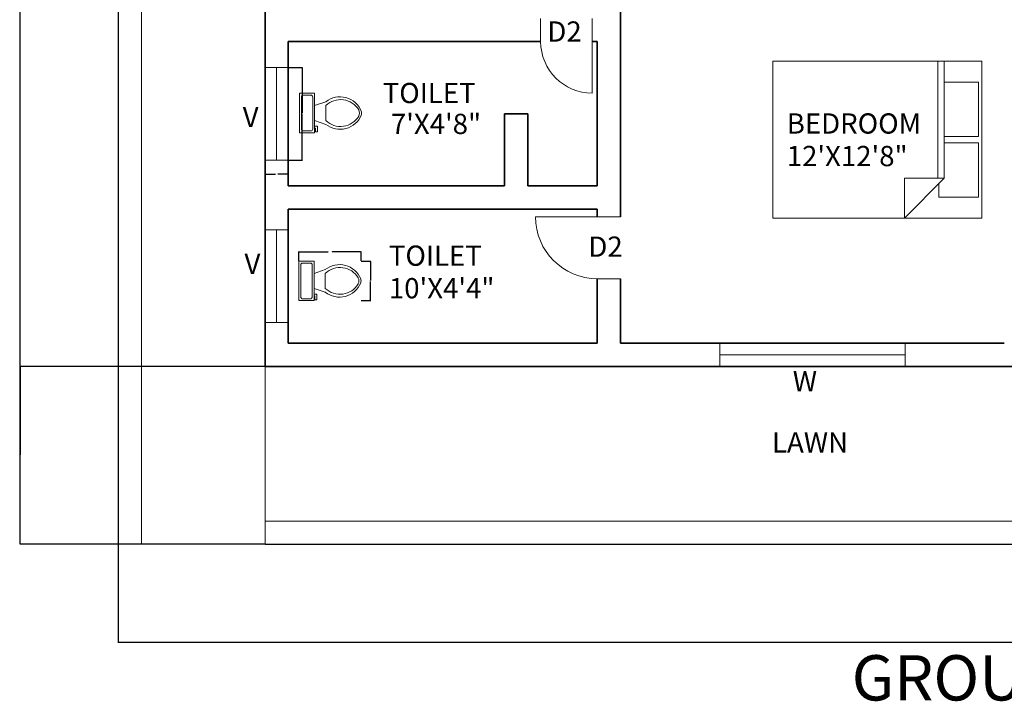
# Model space of a CAD drawing. Units: feet. Extents: x 2219 to 3039, y 1768 to 2369.
# Tile 1 of 16: x 2219 to 2601, y 1768 to 2032. Entities that reach past the tile are written whole.
import ezdxf

# ---------------------------------------------------------------- set-up
doc = ezdxf.new("R2010")
doc.units = ezdxf.units.FT
for name, color, linetype, lineweight in [('A-ANNO-DIMS', 2, 'Continuous', 18), ('A-ANNO-TEXT', 7, 'Continuous', 18), ('A-ANNO-TITL', 7, 'Continuous', 35), ('A-AREA-IDEN', 7, 'Continuous', 18), ('A-DOOR', 4, 'Continuous', 20), ('A-FLOR-FIXT', 9, 'Continuous', 18), ('A-FURN', 8, 'Continuous', 18), ('A-GLAZ', 4, 'Continuous', 18), ('A-WALL', 7, 'Continuous', 35), ('C-PROP', 7, 'Continuous', 30), ('C-SITE', 3, 'Continuous', 20)]:
    doc.layers.add(name, color=color, linetype=linetype, lineweight=lineweight)
doc.styles.get("Standard").update_dxf_attribs({"font": 'arial.ttf'})
doc.dimstyles.get("Standard").update_dxf_attribs({"dimtxt": 0.18, "dimasz": 0.18, "dimexe": 0.18, "dimexo": 0.0625, "dimgap": 0.09, "dimtad": 0, "dimtih": 1, "dimtoh": 1, "dimdec": 4, "dimzin": 0, "dimdsep": 46, "dimtxsty": 'Standard', "dimcen": 0.09, "dimadec": 0, "dimazin": 0, "dimtfac": 1, "dimtdec": 4, "dimtofl": 0, "dimtmove": 0, "dimatfit": 3, "dimfxl": 1, "dimtolj": 1, "dimtzin": 0, "dimarcsym": 0})

# ---------------------------------------------------------------- blocks, each defined once
blk = doc.blocks.new('Bed - Queen')
for p, q in [((0, -80.00003), (0, 0)), ((0, 0), (59.99999, 0)), ((59.99999, 0), (59.99999, -80.00003)), ((7.99999, -1.2), (28.79998, -1.2)), ((7.99999, -14.4), (7.99999, -1.2)), ((28.79998, -1.2), (28.79998, -14.4)), ((31.19999, -1.2), (51.99999, -1.2)), ((31.19999, -14.4), (31.19999, -1.2)), ((51.99999, -1.2), (51.99999, -16.4)), ((0, -14.4), (44.8, -14.4)), ((59.99999, -29.6), (44.8, -14.4)), ((44.8, -14.4), (44.8, -29.6)), ((44.8, -16.8), (0, -16.8)), ((51.99999, -16.4), (46.79936, -16.4)), ((44.8, -29.6), (59.99999, -29.6)), ((59.99999, -80.00003), (0, -80.00003))]:
    blk.add_line(p, q)
blk = doc.blocks.new('Toilet - top')
for p, q in [((9.5, -6), (9.5, -2)), ((-10, -8.5), (-8, -8.5)), ((-10, -9.5), (-10, -8.5)), ((-7, -9.5), (-10, -9.5)), ((-8, -8.5), (-8, -8)), ((-7, -8), (-7, -9.5)), ((-4, -8), (-6, -14)), ((4, -8), (6, -14)), ((4, -14), (-4, -14))]:
    blk.add_line(p, q)
blk.add_lwpolyline([(10.5, -8), (10.5, 0), (-10.5, 0), (-10.5, -8)], close=True)
for points in [[(-9.5, -2), (-9.5, -6)], [(8.5, -1), (-8.5, -1)], [(-8.5, -7), (8.5, -7)]]:
    blk.add_lwpolyline(points)
for centre, radius, start, end in [((-8.62, -1.88), 0.884, 81.8699, 188.1301), ((8.62, -1.88), 0.884, 351.8699, 98.1301), ((-8.62, -6.12), 0.884, 171.8699, 278.1301), ((8.62, -6.12), 0.884, 261.8699, 8.1301), ((3.52, -21.58), 12.17, 141.4691, 247.9714), ((4.2, -21.82), 11.33, 136.3677, 238.9468), ((-3.52, -21.58), 12.17, 292.0284, 38.5307), ((-4.2, -21.82), 11.33, 301.053, 43.6321), ((0, -27.88), 4, 245.7318, 294.2682), ((0, -29), 4, 254.8605, 285.1395)]:
    blk.add_arc(centre, radius, start, end)
blk = doc.blocks.new('DOOR-24-INTEGRAL-JAMB')
for p, q in [((9, 24), (0, 24)), ((33, 0), (0, 0))]:
    blk.add_line(p, q)
blk.add_arc((9, 0), 24, 0, 90)
blk = doc.blocks.new('DOOR-20')
for p, q in [((0, 29), (0, 0)), ((20, 9), (20, 0))]:
    blk.add_line(p, q)
blk.add_arc((0, 9), 20, 0, 90)
blk = doc.blocks.new('WINDOW-72')
for p, q in [((9, 72), (0, 72)), ((4.5, 72), (4.5, 0)), ((9, 0), (0, 0))]:
    blk.add_line(p, q)
blk = doc.blocks.new('VENT-WINDOW-36')
for p, q in [((0, 36), (9, 36)), ((4.5, 36), (4.5, 0)), ((0, 0), (9, 0))]:
    blk.add_line(p, q)
blk = doc.blocks.new('*D18')
at = {"layer": 'A-ANNO-DIMS', "color": 0, "lineweight": -2, "transparency": 16777216}
for p, q in [((2327.57, 1938.8), (2327.57, 1942.54)), ((2327.75, 1942.36), (2338.85, 1942.36)), ((2351.5, 1942.36), (2340.4, 1942.36)), ((2351.68, 1938.8), (2351.68, 1942.54))]:
    blk.add_line(p, q, dxfattribs=at)
at = {"layer": 'A-ANNO-DIMS', "color": 0, "transparency": 16777216}
for points in [[(2327.75, 1942.39), (2327.75, 1942.33), (2327.57, 1942.36)], [(2351.5, 1942.39), (2351.5, 1942.33), (2351.68, 1942.36)]]:
    blk.add_solid(points, dxfattribs=at)
at = {"layer": 'Defpoints', "color": 0, "transparency": 16777216}
for p in [(2327.57, 1942.36), (2327.57, 1938.74), (2351.68, 1938.74)]:
    blk.add_point(p, dxfattribs=at)
at = {"layer": 'A-ANNO-DIMS', "color": 0, "transparency": 16777216, "insert": (2339.63, 1942.36), "char_height": 0.18, "attachment_point": 5}
blk.add_mtext('\\A1;WC 24 TYP.', dxfattribs=at)
blk = doc.blocks.new('*D19')
at = {"layer": 'A-ANNO-DIMS', "color": 0, "lineweight": -2, "transparency": 16777216}
for p, q in [((2351.75, 1938.74), (2355.48, 1938.74)), ((2355.3, 1938.56), (2355.3, 1931.26)), ((2355.3, 1923.6), (2355.3, 1930.9)), ((2351.75, 1923.42), (2355.48, 1923.42))]:
    blk.add_line(p, q, dxfattribs=at)
at = {"layer": 'A-ANNO-DIMS', "color": 0, "transparency": 16777216}
for points in [[(2355.27, 1938.56), (2355.33, 1938.56), (2355.3, 1938.74)], [(2355.27, 1923.6), (2355.33, 1923.6), (2355.3, 1923.42)]]:
    blk.add_solid(points, dxfattribs=at)
at = {"layer": 'Defpoints', "color": 0, "transparency": 16777216}
for p in [(2351.68, 1938.74), (2355.3, 1938.74), (2351.68, 1923.42)]:
    blk.add_point(p, dxfattribs=at)
at = {"layer": 'A-ANNO-DIMS', "color": 0, "transparency": 16777216, "insert": (2355.3, 1931.08), "char_height": 0.18, "attachment_point": 5}
blk.add_mtext('\\A1;15 TYP.', dxfattribs=at)
blk = doc.blocks.new('*D38')
at = {"layer": 'A-ANNO-DIMS', "color": 0, "lineweight": -2, "transparency": 16777216}
for p, q in [((2323.46, 2013.92), (2328.98, 2013.92)), ((2328.8, 2013.74), (2328.8, 1996.11)), ((2328.8, 1978.1), (2328.8, 1995.74)), ((2323.46, 1977.92), (2328.98, 1977.92))]:
    blk.add_line(p, q, dxfattribs=at)
at = {"layer": 'A-ANNO-DIMS', "color": 0, "transparency": 16777216}
for points in [[(2328.77, 2013.74), (2328.83, 2013.74), (2328.8, 2013.92)], [(2328.77, 1978.1), (2328.83, 1978.1), (2328.8, 1977.92)]]:
    blk.add_solid(points, dxfattribs=at)
at = {"layer": 'Defpoints', "color": 0, "transparency": 16777216}
for p in [(2323.4, 2013.92), (2328.8, 2013.92), (2323.4, 1977.92)]:
    blk.add_point(p, dxfattribs=at)
at = {"layer": 'A-ANNO-DIMS', "color": 0, "transparency": 16777216, "insert": (2328.8, 1995.92), "char_height": 0.18, "attachment_point": 5}
blk.add_mtext('\\A1;VENT WINDOW 36 TYP.', dxfattribs=at)
blk = doc.blocks.new('*D39')
at = {"layer": 'A-ANNO-DIMS', "color": 0, "lineweight": -2, "transparency": 16777216}
for p, q in [((2314.4, 1977.86), (2314.4, 1972.34)), ((2323.4, 1977.86), (2323.4, 1972.34)), ((2314.58, 1972.52), (2318.44, 1972.52)), ((2323.22, 1972.52), (2319.36, 1972.52))]:
    blk.add_line(p, q, dxfattribs=at)
at = {"layer": 'A-ANNO-DIMS', "color": 0, "transparency": 16777216}
for points in [[(2314.58, 1972.55), (2314.58, 1972.49), (2314.4, 1972.52)], [(2323.22, 1972.55), (2323.22, 1972.49), (2323.4, 1972.52)]]:
    blk.add_solid(points, dxfattribs=at)
at = {"layer": 'Defpoints', "color": 0, "transparency": 16777216}
for p in [(2314.4, 1977.92), (2323.4, 1977.92), (2323.4, 1972.52)]:
    blk.add_point(p, dxfattribs=at)
at = {"layer": 'A-ANNO-DIMS', "color": 0, "transparency": 16777216, "insert": (2318.9, 1972.52), "char_height": 0.18, "attachment_point": 5}
blk.add_mtext('\\A1;9 TYP.', dxfattribs=at)
blk = doc.blocks.new('*D46')
at = {"layer": 'A-ANNO-DIMS', "color": 0, "lineweight": -2, "transparency": 16777216}
for p, q in [((2257.4, 1828.86), (2257.4, 1790.69)), ((3000.4, 1828.86), (3000.4, 1790.69)), ((2257.58, 1790.87), (2628.61, 1790.87)), ((3000.22, 1790.87), (2629.19, 1790.87))]:
    blk.add_line(p, q, dxfattribs=at)
at = {"layer": 'A-ANNO-DIMS', "color": 0, "transparency": 16777216}
for points in [[(2257.58, 1790.9), (2257.58, 1790.84), (2257.4, 1790.87)], [(3000.22, 1790.9), (3000.22, 1790.84), (3000.4, 1790.87)]]:
    blk.add_solid(points, dxfattribs=at)
at = {"layer": 'Defpoints', "color": 0, "transparency": 16777216}
for p in [(2257.4, 1828.92), (3000.4, 1828.92), (3000.4, 1790.87)]:
    blk.add_point(p, dxfattribs=at)
at = {"layer": 'A-ANNO-DIMS', "color": 0, "transparency": 16777216, "insert": (2628.9, 1790.87), "char_height": 0.18, "attachment_point": 5}
blk.add_mtext('\\A1;743', dxfattribs=at)
blk = doc.blocks.new('*D47')
at = {"layer": 'A-ANNO-DIMS', "color": 0, "lineweight": -2, "transparency": 16777216}
for p, q in [((2257.34, 2330.92), (2219.17, 2330.92)), ((2219.35, 2330.74), (2219.35, 2080.1)), ((2219.35, 1829.1), (2219.35, 2079.74)), ((2257.34, 1828.92), (2219.17, 1828.92))]:
    blk.add_line(p, q, dxfattribs=at)
at = {"layer": 'A-ANNO-DIMS', "color": 0, "transparency": 16777216}
for points in [[(2219.32, 2330.74), (2219.38, 2330.74), (2219.35, 2330.92)], [(2219.32, 1829.1), (2219.38, 1829.1), (2219.35, 1828.92)]]:
    blk.add_solid(points, dxfattribs=at)
at = {"layer": 'Defpoints', "color": 0, "transparency": 16777216}
for p in [(2219.35, 2330.92), (2257.4, 2330.92), (2257.4, 1828.92)]:
    blk.add_point(p, dxfattribs=at)
at = {"layer": 'A-ANNO-DIMS', "color": 0, "transparency": 16777216, "insert": (2219.35, 2079.92), "char_height": 0.18, "attachment_point": 5}
blk.add_mtext('\\A1;502', dxfattribs=at)
blk = doc.blocks.new('*D48')
at = {"layer": 'A-ANNO-DIMS', "color": 0, "lineweight": -2, "transparency": 16777216}
for p, q in [((2314.34, 1897.92), (2219.17, 1897.92)), ((2219.35, 1897.74), (2219.35, 1863.6)), ((2219.35, 1829.1), (2219.35, 1863.24)), ((2314.34, 1828.92), (2219.17, 1828.92))]:
    blk.add_line(p, q, dxfattribs=at)
at = {"layer": 'A-ANNO-DIMS', "color": 0, "transparency": 16777216}
for points in [[(2219.32, 1897.74), (2219.38, 1897.74), (2219.35, 1897.92)], [(2219.32, 1829.1), (2219.38, 1829.1), (2219.35, 1828.92)]]:
    blk.add_solid(points, dxfattribs=at)
at = {"layer": 'Defpoints', "color": 0, "transparency": 16777216}
for p in [(2219.35, 1897.92), (2314.4, 1897.92), (2314.4, 1828.92)]:
    blk.add_point(p, dxfattribs=at)
at = {"layer": 'A-ANNO-DIMS', "color": 0, "transparency": 16777216, "insert": (2219.35, 1863.42), "char_height": 0.18, "attachment_point": 5}
blk.add_mtext('\\A1;69', dxfattribs=at)

msp = doc.modelspace()

# ---------------------------------------------------------------- linework, layer by layer
at = {"layer": 'A-GLAZ'}
msp.add_line((2526.9, 1897.923), (2490.9, 1897.923), dxfattribs=at)
at = {"layer": 'A-WALL'}
for p, q in [((2314.4, 1897.923), (2314.4, 2196.923)), ((2452.4, 1955.923), (2452.4, 2058.923)), ((2314.4, 2023.923), (2314.4, 1967.923)), ((2323.4, 2023.923), (2416.4, 2023.923)), ((2323.4, 2023.923), (2323.4, 1967.923)), ((2416.4, 2023.923), (2421.4, 2023.923)), ((2441.4, 2023.923), (2443.4, 2023.923)), ((2443.4, 2023.923), (2443.4, 1967.923)), ((2452.4, 2023.923), (2452.4, 1967.923)), ((2407.4, 1967.923), (2407.4, 1995.923)), ((2416.4, 1995.923), (2407.4, 1995.923)), ((2416.4, 1967.923), (2416.4, 1995.923)), ((2323.4, 1967.923), (2407.4, 1967.923)), ((2443.4, 1967.923), (2416.4, 1967.923)), ((2314.4, 1958.923), (2314.4, 1897.923)), ((2323.4, 1958.923), (2443.4, 1958.923)), ((2323.4, 1958.923), (2323.4, 1906.923)), ((2443.4, 1958.923), (2416.4, 1958.923)), ((2443.4, 1955.923), (2443.4, 1958.923)), ((2452.4, 1955.923), (2452.4, 1958.923)), ((2443.4, 1906.923), (2443.4, 1931.923)), ((2452.4, 1906.923), (2452.4, 1931.923)), ((2452.4, 1906.923), (2452.4, 1931.923)), ((2323.4, 1906.923), (2443.4, 1906.923)), ((2452.4, 1906.923), (2601.4, 1906.923)), ((2314.4, 1897.923), (2443.4, 1897.923)), ((2610.4, 1897.923), (2443.4, 1897.923))]:
    msp.add_line(p, q, dxfattribs=at)
at = {"layer": 'C-PROP'}
for p, q in [((2257.4, 2330.923), (2257.4, 1828.923)), ((2314.4, 1828.923), (2257.4, 1828.923)), ((2314.4, 1828.923), (3000.4, 1828.923))]:
    msp.add_line(p, q, dxfattribs=at)
at = {"layer": 'C-SITE'}
for p, q in [((2266.4, 2319.623), (2266.4, 1828.923)), ((2314.4, 1897.923), (2314.4, 1828.923)), ((2314.4, 1837.923), (2763.4, 1837.923))]:
    msp.add_line(p, q, dxfattribs=at)

# ---------------------------------------------------------------- block references
at = {"layer": 'A-DOOR', "rotation": 180}
for name, p in [('DOOR-20', (2441.399, 2032.922)), ('DOOR-24-INTEGRAL-JAMB', (2452.399, 1955.922))]:
    msp.add_blockref(name, p, dxfattribs=at)
at = {"layer": 'A-FLOR-FIXT', "xscale": 0.7296686166335911, "yscale": 0.7296686166335911, "zscale": 0.7296686166335911, "rotation": 90}
for p in [(2327.792, 1996.186), (2327.572, 1931.077)]:
    msp.add_blockref('Toilet - top', p, dxfattribs=at)
at = {"layer": 'A-FURN', "xscale": 1.013648725183241, "yscale": 1.013648725183241, "zscale": 1.013648725183241, "rotation": 270}
msp.add_blockref('Bed - Queen', (2592.616, 2016.286), dxfattribs=at)
at = {"layer": 'A-GLAZ'}
for p in [(2314.4, 1977.923), (2314.4, 1914.923)]:
    msp.add_blockref('VENT-WINDOW-36', p, dxfattribs=at)
at = {"layer": 'A-GLAZ', "rotation": 90.0000000000009}
msp.add_blockref('WINDOW-72', (2562.899, 1897.923), dxfattribs=at)

# ---------------------------------------------------------------- texts
at = {"layer": 'A-ANNO-TEXT'}
for s, height, p in [('D2', 7.8584, (2423.991, 2023.89)), ('V', 7.858, (2305.723, 1990.731)), ('D2', 7.8584, (2439.919, 1940.43)), ('V', 7.858, (2306.416, 1933.767)), ('W', 7.858, (2519.276, 1888.221))]:
    msp.add_text(s, height=height, dxfattribs=at).set_placement(p)
at = {"layer": 'A-ANNO-TITL'}
msp.add_text('GROUND FLOOR', height=17.56585, dxfattribs=at).set_placement((2542.155, 1768.289))
at = {"layer": 'A-AREA-IDEN'}
for s, p in [('TOILET', (2360.07, 2000.035)), ('7\'X4\'8"', (2363.249, 1988.047)), ('BEDROOM', (2516.934, 1988.209)), ('12\'X12\'8"', (2516.934, 1975.585)), ('TOILET', (2362.474, 1936.935)), ('10\'X4\'4"', (2362.474, 1924.311)), ('LAWN', (2511.219, 1864.497))]:
    msp.add_text(s, height=7.8584, dxfattribs=at).set_placement(p)

# ---------------------------------------------------------------- dimensions: what is measured, and where the dimension line sits
at = {"layer": 'A-ANNO-DIMS'}
for base, p1, p2, picture, middle in [((2219.35, 2330.923), (2257.4, 1828.923), (2257.4, 2330.923), '*D47', (2219.35, 2079.923)), ((2219.35, 1897.923), (2314.4, 1828.923), (2314.4, 1897.923), '*D48', (2219.35, 1863.423))]:
    dim = msp.add_linear_dim(base=base, p1=p1, p2=p2, angle=90, dimstyle='Standard', override={"dimdec": 0, "dimlfac": 1, "dimrnd": 0, "dimzin": 0, "dimdsep": 46, "dimlunit": 2}, dxfattribs=at)
    dim.commit()
    dim.dimension.update_dxf_attribs({"geometry": picture, "text_midpoint": middle})
for base, p1, p2, angle, text, picture, middle in [((2328.8, 2013.923), (2323.4, 1977.923), (2323.4, 2013.923), 90, 'VENT WINDOW <> TYP.', '*D38', (2328.8, 1995.923)), ((2327.572, 1942.356), (2351.685, 1938.739), (2327.572, 1938.739), 180, 'WC <> TYP.', '*D18', (2339.628, 1942.356)), ((2355.301, 1938.739), (2351.685, 1923.416), (2351.685, 1938.739), 90, '<> TYP.', '*D19', (2355.301, 1931.077))]:
    dim = msp.add_linear_dim(base=base, p1=p1, p2=p2, angle=angle, text=text, dimstyle='Standard', override={"dimdec": 0, "dimlfac": 1, "dimrnd": 0, "dimzin": 0, "dimdsep": 46, "dimlunit": 2}, dxfattribs=at)
    dim.commit()
    dim.dimension.update_dxf_attribs({"geometry": picture, "text_midpoint": middle})
dim = msp.add_linear_dim(base=(2323.4, 1972.523), p1=(2314.4, 1977.923), p2=(2323.4, 1977.923), text='<> TYP.', dimstyle='Standard', override={"dimdec": 0, "dimlfac": 1, "dimrnd": 0, "dimzin": 0, "dimdsep": 46, "dimlunit": 2}, dxfattribs=at)
dim.commit()
dim.dimension.update_dxf_attribs({"geometry": '*D39', "text_midpoint": (2318.9, 1972.523)})
dim = msp.add_linear_dim(base=(3000.4, 1790.873), p1=(2257.4, 1828.923), p2=(3000.4, 1828.923), dimstyle='Standard', override={"dimdec": 0, "dimlfac": 1, "dimrnd": 0, "dimzin": 0, "dimdsep": 46, "dimlunit": 2}, dxfattribs=at)
dim.commit()
dim.dimension.update_dxf_attribs({"geometry": '*D46', "text_midpoint": (2628.9, 1790.873)})

doc.saveas('drawing.dxf')
